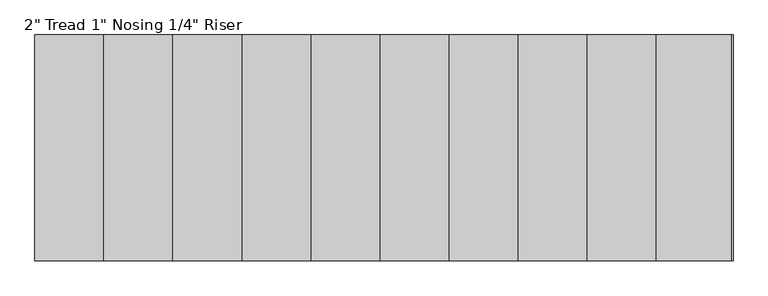
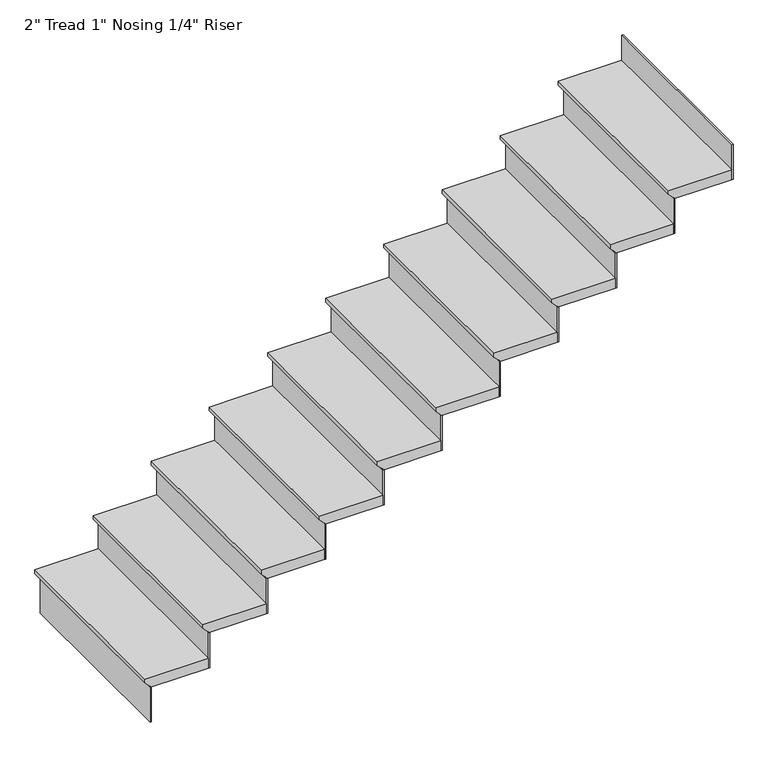
"""IFC4 building model written with IfcOpenShell, lengths in millimetres: stair flight geometry."""

from ifc_helpers import new_model, si_unit, frame, origin, place, context, project, spatial, polyline, outline, extrude, source, transform, mapped, element, save


def stair_flight_b41fd25d(model_context):
    return source(origin(), model_context, "Body", "SweptSolid", [
        extrude(outline(polyline([(2032.0, -7947.6763529), (2032.0, -8252.4763529), (2012.95, -8252.4763529), (1987.55, -8227.0763529), (1981.2, -8227.0763529), (1981.2, -7947.6763529), (2032.0, -7947.6763529)])), frame((0.0, -3490.0338022, 0.0), z_axis=(0.0, 1.0, 0.0), x_axis=(0.0, 0.0, 1.0)), (0.0, 0.0, 1.0), 914.4),
        extrude(outline(polyline([(-8220.7263529, -3490.0338022), (-8227.0763529, -3490.0338022), (-8227.0763529, -2575.6338022), (-8220.7263529, -2575.6338022), (-8220.7263529, -3490.0338022)])), frame((0.0, 0.0, 1803.4), z_axis=(0.0, 0.0, 1.0), x_axis=(1.0, 0.0, 0.0)), (0.0, 0.0, 1.0), 177.8),
        extrude(outline(polyline([(-7941.3263529, -3490.0338022), (-7947.6763529, -3490.0338022), (-7947.6763529, -2575.6338022), (-7941.3263529, -2575.6338022), (-7941.3263529, -3490.0338022)])), frame((0.0, 0.0, 1981.2), z_axis=(0.0, 0.0, 1.0), x_axis=(1.0, 0.0, 0.0)), (0.0, 0.0, 1.0), 177.8),
        extrude(outline(polyline([(2209.8, -7668.2763529), (2209.8, -7973.0763529), (2190.75, -7973.0763529), (2165.35, -7947.6763529), (2159.0, -7947.6763529), (2159.0, -7668.2763529), (2209.8, -7668.2763529)])), frame((0.0, -3490.0338022, 0.0), z_axis=(0.0, 1.0, 0.0), x_axis=(0.0, 0.0, 1.0)), (0.0, 0.0, 1.0), 914.4),
        extrude(outline(polyline([(-7661.9263529, -3490.0338022), (-7668.2763529, -3490.0338022), (-7668.2763529, -2575.6338022), (-7661.9263529, -2575.6338022), (-7661.9263529, -3490.0338022)])), frame((0.0, 0.0, 2159.0), z_axis=(0.0, 0.0, 1.0), x_axis=(1.0, 0.0, 0.0)), (0.0, 0.0, 1.0), 177.8),
        extrude(outline(polyline([(2387.6, -7388.8763529), (2387.6, -7693.6763529), (2368.55, -7693.6763529), (2343.15, -7668.2763529), (2336.8, -7668.2763529), (2336.8, -7388.8763529), (2387.6, -7388.8763529)])), frame((0.0, -3490.0338022, 0.0), z_axis=(0.0, 1.0, 0.0), x_axis=(0.0, 0.0, 1.0)), (0.0, 0.0, 1.0), 914.4),
        extrude(outline(polyline([(-7382.5263529, -3490.0338022), (-7388.8763529, -3490.0338022), (-7388.8763529, -2575.6338022), (-7382.5263529, -2575.6338022), (-7382.5263529, -3490.0338022)])), frame((0.0, 0.0, 2336.8), z_axis=(0.0, 0.0, 1.0), x_axis=(1.0, 0.0, 0.0)), (0.0, 0.0, 1.0), 177.8),
        extrude(outline(polyline([(2565.4, -7109.4763529), (2565.4, -7414.2763529), (2546.35, -7414.2763529), (2520.95, -7388.8763529), (2514.6, -7388.8763529), (2514.6, -7109.4763529), (2565.4, -7109.4763529)])), frame((0.0, -3490.0338022, 0.0), z_axis=(0.0, 1.0, 0.0), x_axis=(0.0, 0.0, 1.0)), (0.0, 0.0, 1.0), 914.4),
        extrude(outline(polyline([(-7103.1263529, -3490.0338022), (-7109.4763529, -3490.0338022), (-7109.4763529, -2575.6338022), (-7103.1263529, -2575.6338022), (-7103.1263529, -3490.0338022)])), frame((0.0, 0.0, 2514.6), z_axis=(0.0, 0.0, 1.0), x_axis=(1.0, 0.0, 0.0)), (0.0, 0.0, 1.0), 177.8),
        extrude(outline(polyline([(2743.2, -6830.0763529), (2743.2, -7134.8763529), (2724.15, -7134.8763529), (2698.75, -7109.4763529), (2692.4, -7109.4763529), (2692.4, -6830.0763529), (2743.2, -6830.0763529)])), frame((0.0, -3490.0338022, 0.0), z_axis=(0.0, 1.0, 0.0), x_axis=(0.0, 0.0, 1.0)), (0.0, 0.0, 1.0), 914.4),
        extrude(outline(polyline([(-6823.7263529, -3490.0338022), (-6830.0763529, -3490.0338022), (-6830.0763529, -2575.6338022), (-6823.7263529, -2575.6338022), (-6823.7263529, -3490.0338022)])), frame((0.0, 0.0, 2692.4), z_axis=(0.0, 0.0, 1.0), x_axis=(1.0, 0.0, 0.0)), (0.0, 0.0, 1.0), 177.8),
        extrude(outline(polyline([(2921.0, -6550.6763529), (2921.0, -6855.4763529), (2901.95, -6855.4763529), (2876.55, -6830.0763529), (2870.2, -6830.0763529), (2870.2, -6550.6763529), (2921.0, -6550.6763529)])), frame((0.0, -3490.0338022, 0.0), z_axis=(0.0, 1.0, 0.0), x_axis=(0.0, 0.0, 1.0)), (0.0, 0.0, 1.0), 914.4),
        extrude(outline(polyline([(-6544.3263529, -3490.0338022), (-6550.6763529, -3490.0338022), (-6550.6763529, -2575.6338022), (-6544.3263529, -2575.6338022), (-6544.3263529, -3490.0338022)])), frame((0.0, 0.0, 2870.2), z_axis=(0.0, 0.0, 1.0), x_axis=(1.0, 0.0, 0.0)), (0.0, 0.0, 1.0), 177.8),
        extrude(outline(polyline([(3098.8, -6271.2763529), (3098.8, -6576.0763529), (3079.75, -6576.0763529), (3054.35, -6550.6763529), (3048.0, -6550.6763529), (3048.0, -6271.2763529), (3098.8, -6271.2763529)])), frame((0.0, -3490.0338022, 0.0), z_axis=(0.0, 1.0, 0.0), x_axis=(0.0, 0.0, 1.0)), (0.0, 0.0, 1.0), 914.4),
        extrude(outline(polyline([(-6264.9263529, -3490.0338022), (-6271.2763529, -3490.0338022), (-6271.2763529, -2575.6338022), (-6264.9263529, -2575.6338022), (-6264.9263529, -3490.0338022)])), frame((0.0, 0.0, 3048.0), z_axis=(0.0, 0.0, 1.0), x_axis=(1.0, 0.0, 0.0)), (0.0, 0.0, 1.0), 177.8),
        extrude(outline(polyline([(3276.6, -5991.8763529), (3276.6, -6296.6763529), (3257.55, -6296.6763529), (3232.15, -6271.2763529), (3225.8, -6271.2763529), (3225.8, -5991.8763529), (3276.6, -5991.8763529)])), frame((0.0, -3490.0338022, 0.0), z_axis=(0.0, 1.0, 0.0), x_axis=(0.0, 0.0, 1.0)), (0.0, 0.0, 1.0), 914.4),
        extrude(outline(polyline([(-5985.5263529, -3490.0338022), (-5991.8763529, -3490.0338022), (-5991.8763529, -2575.6338022), (-5985.5263529, -2575.6338022), (-5985.5263529, -3490.0338022)])), frame((0.0, 0.0, 3225.8), z_axis=(0.0, 0.0, 1.0), x_axis=(1.0, 0.0, 0.0)), (0.0, 0.0, 1.0), 177.8),
        extrude(outline(polyline([(3454.4, -5712.4763529), (3454.4, -6017.2763529), (3435.35, -6017.2763529), (3409.95, -5991.8763529), (3403.6, -5991.8763529), (3403.6, -5712.4763529), (3454.4, -5712.4763529)])), frame((0.0, -3490.0338022, 0.0), z_axis=(0.0, 1.0, 0.0), x_axis=(0.0, 0.0, 1.0)), (0.0, 0.0, 1.0), 914.4),
        extrude(outline(polyline([(-5706.1263529, -3490.0338022), (-5712.4763529, -3490.0338022), (-5712.4763529, -2575.6338022), (-5706.1263529, -2575.6338022), (-5706.1263529, -3490.0338022)])), frame((0.0, 0.0, 3403.6), z_axis=(0.0, 0.0, 1.0), x_axis=(1.0, 0.0, 0.0)), (0.0, 0.0, 1.0), 177.8),
        extrude(outline(polyline([(-5426.7263529, -3490.0338022), (-5433.0763529, -3490.0338022), (-5433.0763529, -2575.6338022), (-5426.7263529, -2575.6338022), (-5426.7263529, -3490.0338022)])), frame((0.0, 0.0, 3581.4), z_axis=(0.0, 0.0, 1.0), x_axis=(1.0, 0.0, 0.0)), (0.0, 0.0, 1.0), 177.8),
        extrude(outline(polyline([(3632.2, -5433.0763529), (3632.2, -5737.8763529), (3613.15, -5737.8763529), (3587.75, -5712.4763529), (3581.4, -5712.4763529), (3581.4, -5433.0763529), (3632.2, -5433.0763529)])), frame((0.0, -3490.0338022, 0.0), z_axis=(0.0, 1.0, 0.0), x_axis=(0.0, 0.0, 1.0)), (0.0, 0.0, 1.0), 914.4),
    ])


if __name__ == "__main__":
    model = new_model("IFC4")
    model_context = context("Model", 3, world=origin())
    ifc_project = project(units=[si_unit("LENGTHUNIT", "METRE", prefix="MILLI")], contexts=[model_context])
    site = spatial("IfcSite", under=ifc_project)
    building = spatial("IfcBuilding", under=site)
    placement = place(None, origin())
    stair_flight_shape = stair_flight_b41fd25d(model_context)
    element("IfcStairFlight", 1, ObjectType="2\" Tread 1\" Nosing 1/4\" Riser", at=placement, inside=building, context=model_context, shape_type="MappedRepresentation", body=[
        mapped(stair_flight_shape, transform((0.0, 0.0, 0.0), x_axis=(1.0, 0.0, 0.0), y_axis=(0.0, 1.0, 0.0), z_axis=(0.0, 0.0, 1.0))),
    ])
    save(model, "model.ifc")
